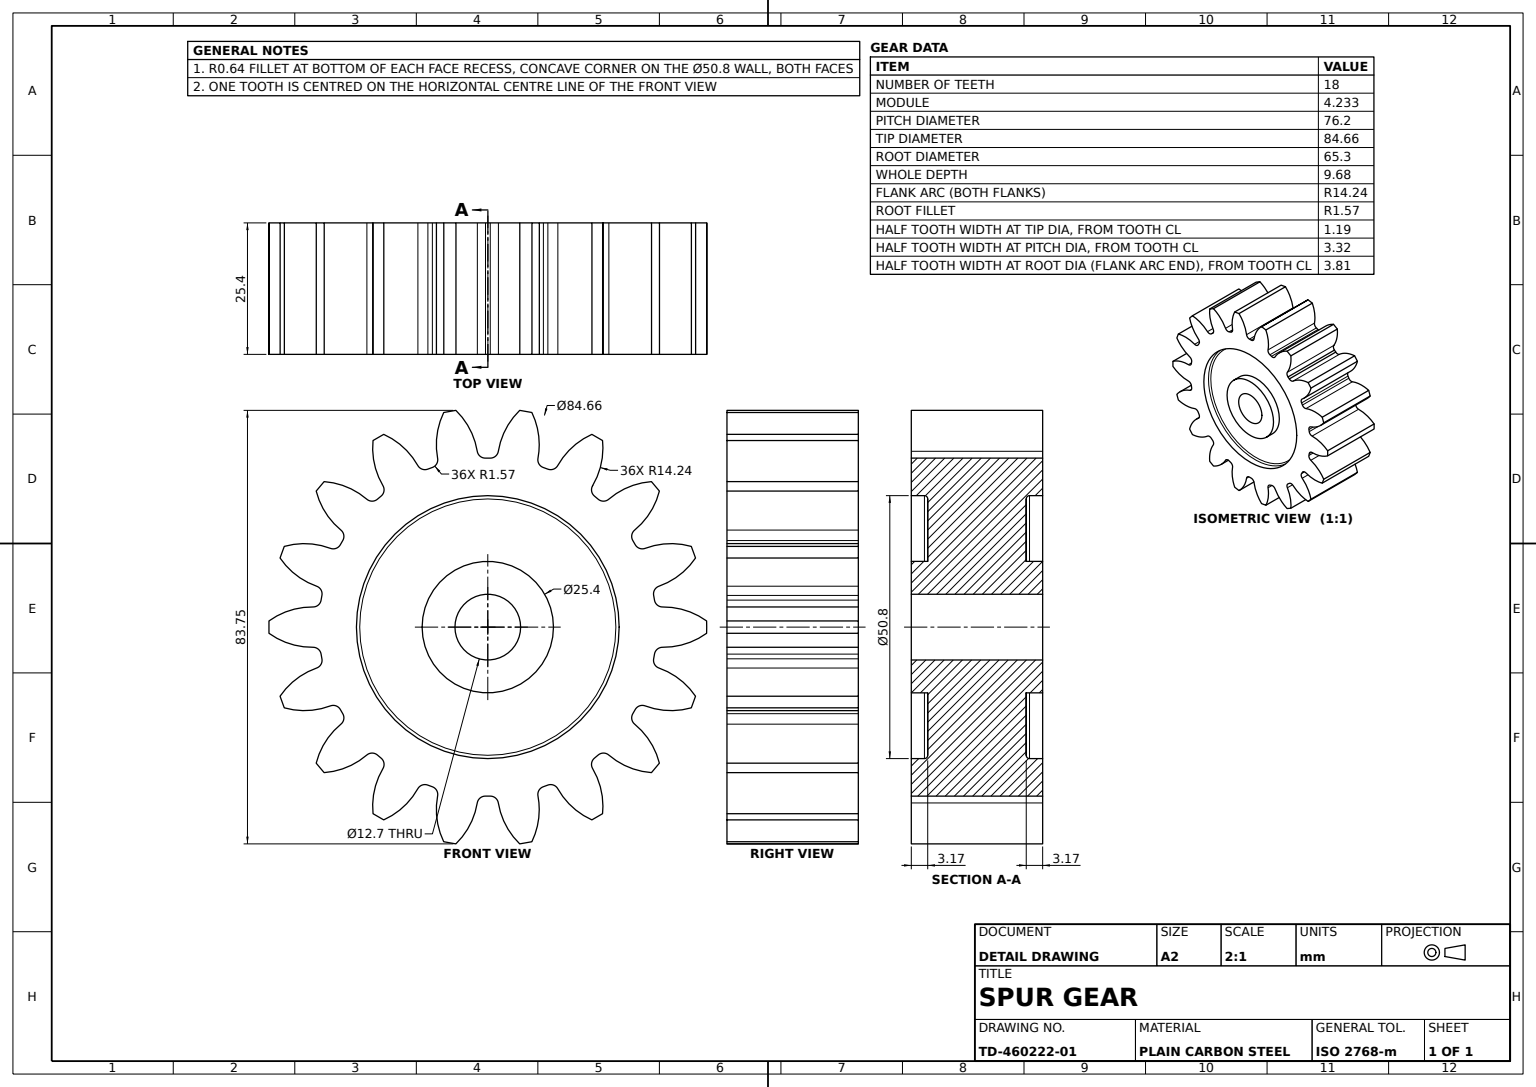
from build123d import *

# Parameters (mm, degrees)
GEAR_PROFILE_18T_SKETCH_R                  = 6.35
GEAR_BODY_18T_DEPTH                        = 12.7
FACE_RECESS_SKETCH_R                       = 25.4
FACE_RECESS_SKETCH_R_2                     = 12.7
FACE_RECESS_0_25IN_DEEP_DEPTH              = 3.175
RECESS_FILLET_R0_025IN_R                   = 0.635
RECESS_FILLET_R0_025IN_OF_FACE_RECESS_MI_R = 0.635


with BuildPart() as part:
    # Gear Profile 18T Sketch → Gear Body 18T (new, symmetric)
    with BuildSketch(Plane.XY):
        with BuildLine():
            ThreePointArc((-42.312262388, 1.1938), (-42.3291, 0), (-42.312262388, -1.1938))
            ThreePointArc((-42.312262388, -1.1938), (-38.27572162, -3.227144912), (-33.805252697, -3.892772818))
            ThreePointArc((-33.805252697, -3.892772818), (-32.773212647, -4.262365971), (-32.232404102, -5.215902483))
            ThreePointArc((-32.232404102, -5.215902483), (-32.155647309, -5.669908203), (-32.072495999, -6.122786396))
            ThreePointArc((-32.072495999, -6.122786396), (-32.254561104, -7.203785037), (-33.09795322, -7.904067481))
            ThreePointArc((-33.09795322, -7.904067481), (-37.071161726, -10.058543535), (-40.168824382, -13.349840996))
            ThreePointArc((-40.168824382, -13.349840996), (-39.776342915, -14.477404849), (-39.352217087, -15.593451097))
            ThreePointArc((-39.352217087, -15.593451097), (-34.863664596, -16.123592054), (-30.435139786, -15.220087264))
            ThreePointArc((-30.435139786, -15.220087264), (-29.338931064, -15.214412737), (-28.50460857, -15.925476545))
            ThreePointArc((-28.50460857, -15.925476545), (-28.277201677, -16.32585), (-28.04417154, -16.722976874))
            ThreePointArc((-28.04417154, -16.722976874), (-27.845533466, -17.801053253), (-28.398552111, -18.74756059))
            ThreePointArc((-28.398552111, -18.74756059), (-31.395272617, -22.131023182), (-33.180433326, -26.283294144))
            ThreePointArc((-33.180433326, -26.283294144), (-32.425971837, -27.208621009), (-31.645713629, -28.112301857))
            ThreePointArc((-31.645713629, -28.112301857), (-27.246535089, -27.075296036), (-23.394099842, -24.711634561))
            ThreePointArc((-23.394099842, -24.711634561), (-22.365941397, -24.331376786), (-21.338736561, -24.7142031))
            ThreePointArc((-21.338736561, -24.7142031), (-20.988108195, -25.012653343), (-20.633306105, -25.306129536))
            ThreePointArc((-20.633306105, -25.306129536), (-20.077923535, -26.251251731), (-20.2738665, -27.329821208))
            ThreePointArc((-20.2738665, -27.329821208), (-21.932650285, -31.534174815), (-22.189992321, -36.046594119))
            ThreePointArc((-22.189992321, -36.046594119), (-21.16455, -36.658075919), (-20.122270067, -37.240394119))
            ThreePointArc((-20.122270067, -37.240394119), (-16.343071335, -34.761319727), (-13.531386197, -31.222594026))
            ThreePointArc((-13.531386197, -31.222594026), (-12.695289112, -30.513617701), (-11.599097997, -30.522032019))
            ThreePointArc((-11.599097997, -30.522032019), (-11.167539114, -30.682561546), (-10.733759438, -30.836989497))
            ThreePointArc((-10.733759438, -30.836989497), (-9.888619707, -31.535161823), (-9.703853378, -32.615702042))
            ThreePointArc((-9.703853378, -32.615702042), (-9.824626637, -37.13383957), (-8.523110752, -41.462142852))
            ThreePointArc((-8.523110752, -41.462142852), (-7.350371077, -41.686025858), (-6.171783761, -41.876745241))
            ThreePointArc((-6.171783761, -41.876745241), (-3.468391979, -38.254615236), (-2.036587675, -33.967647854))
            ThreePointArc((-2.036587675, -33.967647854), (-1.493397598, -33.015465989), (-0.46043703, -32.648453419))
            ThreePointArc((-0.46043703, -32.648453419), (0, -32.6517), (0.46043703, -32.648453419))
            ThreePointArc((0.46043703, -32.648453419), (1.493397598, -33.015465989), (2.036587675, -33.967647854))
            ThreePointArc((2.036587675, -33.967647854), (3.468391979, -38.254615236), (6.171783761, -41.876745241))
            ThreePointArc((6.171783761, -41.876745241), (7.350371077, -41.686025858), (8.523110752, -41.462142852))
            ThreePointArc((8.523110752, -41.462142852), (9.824626637, -37.13383957), (9.703853378, -32.615702042))
            ThreePointArc((9.703853378, -32.615702042), (9.888619707, -31.535161823), (10.733759438, -30.836989497))
            ThreePointArc((10.733759438, -30.836989497), (11.167539114, -30.682561546), (11.599097997, -30.522032019))
            ThreePointArc((11.599097997, -30.522032019), (12.695289112, -30.513617701), (13.531386197, -31.222594026))
            ThreePointArc((13.531386197, -31.222594026), (16.343071335, -34.761319727), (20.122270067, -37.240394119))
            ThreePointArc((20.122270067, -37.240394119), (21.16455, -36.658075919), (22.189992321, -36.046594119))
            ThreePointArc((22.189992321, -36.046594119), (21.932650285, -31.534174815), (20.2738665, -27.329821208))
            ThreePointArc((20.2738665, -27.329821208), (20.077923535, -26.251251731), (20.633306105, -25.306129536))
            ThreePointArc((20.633306105, -25.306129536), (20.988108195, -25.012653343), (21.338736561, -24.7142031))
            ThreePointArc((21.338736561, -24.7142031), (22.365941397, -24.331376786), (23.394099842, -24.711634561))
            ThreePointArc((23.394099842, -24.711634561), (27.246535089, -27.075296036), (31.645713629, -28.112301857))
            ThreePointArc((31.645713629, -28.112301857), (32.425971837, -27.208621009), (33.180433326, -26.283294144))
            ThreePointArc((33.180433326, -26.283294144), (31.395272617, -22.131023182), (28.398552111, -18.74756059))
            ThreePointArc((28.398552111, -18.74756059), (27.845533466, -17.801053253), (28.04417154, -16.722976874))
            ThreePointArc((28.04417154, -16.722976874), (28.277201677, -16.32585), (28.50460857, -15.925476545))
            ThreePointArc((28.50460857, -15.925476545), (29.338931064, -15.214412737), (30.435139786, -15.220087264))
            ThreePointArc((30.435139786, -15.220087264), (34.863664596, -16.123592054), (39.352217087, -15.593451097))
            ThreePointArc((39.352217087, -15.593451097), (39.776342915, -14.477404849), (40.168824382, -13.349840996))
            ThreePointArc((40.168824382, -13.349840996), (37.071161726, -10.058543535), (33.09795322, -7.904067481))
            ThreePointArc((33.09795322, -7.904067481), (32.254561104, -7.203785037), (32.072495999, -6.122786396))
            ThreePointArc((32.072495999, -6.122786396), (32.155647309, -5.669908203), (32.232404102, -5.215902483))
            ThreePointArc((32.232404102, -5.215902483), (32.773212647, -4.262365971), (33.805252697, -3.892772818))
            ThreePointArc((33.805252697, -3.892772818), (38.27572162, -3.227144912), (42.312262388, -1.1938))
            ThreePointArc((42.312262388, -1.1938), (42.3291, 0), (42.312262388, 1.1938))
            ThreePointArc((42.312262388, 1.1938), (38.27572162, 3.227144912), (33.805252697, 3.892772818))
            ThreePointArc((33.805252697, 3.892772818), (32.773212647, 4.262365971), (32.232404102, 5.215902483))
            ThreePointArc((32.232404102, 5.215902483), (32.155647309, 5.669908203), (32.072495999, 6.122786396))
            ThreePointArc((32.072495999, 6.122786396), (32.254561104, 7.203785037), (33.09795322, 7.904067481))
            ThreePointArc((33.09795322, 7.904067481), (37.071161726, 10.058543535), (40.168824382, 13.349840996))
            ThreePointArc((40.168824382, 13.349840996), (39.776342915, 14.477404849), (39.352217087, 15.593451097))
            ThreePointArc((39.352217087, 15.593451097), (34.863664596, 16.123592054), (30.435139786, 15.220087264))
            ThreePointArc((30.435139786, 15.220087264), (29.338931064, 15.214412737), (28.50460857, 15.925476545))
            ThreePointArc((28.50460857, 15.925476545), (28.277201677, 16.32585), (28.04417154, 16.722976874))
            ThreePointArc((28.04417154, 16.722976874), (27.845533466, 17.801053253), (28.398552111, 18.74756059))
            ThreePointArc((28.398552111, 18.74756059), (31.395272617, 22.131023182), (33.180433326, 26.283294144))
            ThreePointArc((33.180433326, 26.283294144), (32.425971837, 27.208621009), (31.645713629, 28.112301857))
            ThreePointArc((31.645713629, 28.112301857), (27.246535089, 27.075296036), (23.394099842, 24.711634561))
            ThreePointArc((23.394099842, 24.711634561), (22.365941397, 24.331376786), (21.338736561, 24.7142031))
            ThreePointArc((21.338736561, 24.7142031), (20.988108195, 25.012653343), (20.633306105, 25.306129536))
            ThreePointArc((20.633306105, 25.306129536), (20.077923535, 26.251251731), (20.2738665, 27.329821208))
            ThreePointArc((20.2738665, 27.329821208), (21.932650285, 31.534174815), (22.189992321, 36.046594119))
            ThreePointArc((22.189992321, 36.046594119), (21.16455, 36.658075919), (20.122270067, 37.240394119))
            ThreePointArc((20.122270067, 37.240394119), (16.343071335, 34.761319727), (13.531386197, 31.222594026))
            ThreePointArc((13.531386197, 31.222594026), (12.695289112, 30.513617701), (11.599097997, 30.522032019))
            ThreePointArc((11.599097997, 30.522032019), (11.167539114, 30.682561546), (10.733759438, 30.836989497))
            ThreePointArc((10.733759438, 30.836989497), (9.888619707, 31.535161823), (9.703853378, 32.615702042))
            ThreePointArc((9.703853378, 32.615702042), (9.824626637, 37.13383957), (8.523110752, 41.462142852))
            ThreePointArc((8.523110752, 41.462142852), (7.350371077, 41.686025858), (6.171783761, 41.876745241))
            ThreePointArc((6.171783761, 41.876745241), (3.468391979, 38.254615236), (2.036587675, 33.967647854))
            ThreePointArc((2.036587675, 33.967647854), (1.493397598, 33.015465989), (0.46043703, 32.648453419))
            ThreePointArc((0.46043703, 32.648453419), (0, 32.6517), (-0.46043703, 32.648453419))
            ThreePointArc((-0.46043703, 32.648453419), (-1.493397598, 33.015465989), (-2.036587675, 33.967647854))
            ThreePointArc((-2.036587675, 33.967647854), (-3.468391979, 38.254615236), (-6.171783761, 41.876745241))
            ThreePointArc((-6.171783761, 41.876745241), (-7.350371077, 41.686025858), (-8.523110752, 41.462142852))
            ThreePointArc((-8.523110752, 41.462142852), (-9.824626637, 37.13383957), (-9.703853378, 32.615702042))
            ThreePointArc((-9.703853378, 32.615702042), (-9.888619707, 31.535161823), (-10.733759438, 30.836989497))
            ThreePointArc((-10.733759438, 30.836989497), (-11.167539114, 30.682561546), (-11.599097997, 30.522032019))
            ThreePointArc((-11.599097997, 30.522032019), (-12.695289112, 30.513617701), (-13.531386197, 31.222594026))
            ThreePointArc((-13.531386197, 31.222594026), (-16.343071335, 34.761319727), (-20.122270067, 37.240394119))
            ThreePointArc((-20.122270067, 37.240394119), (-21.16455, 36.658075919), (-22.189992321, 36.046594119))
            ThreePointArc((-22.189992321, 36.046594119), (-21.932650285, 31.534174815), (-20.2738665, 27.329821208))
            ThreePointArc((-20.2738665, 27.329821208), (-20.077923535, 26.251251731), (-20.633306105, 25.306129536))
            Line((-20.633306105, 25.306129536), (-21.338736561, 24.7142031))
            ThreePointArc((-21.338736561, 24.7142031), (-22.365941397, 24.331376786), (-23.394099842, 24.711634561))
            ThreePointArc((-23.394099842, 24.711634561), (-27.246535089, 27.075296036), (-31.645713629, 28.112301857))
            ThreePointArc((-31.645713629, 28.112301857), (-32.425971837, 27.208621009), (-33.180433326, 26.283294144))
            ThreePointArc((-33.180433326, 26.283294144), (-31.395272617, 22.131023182), (-28.398552111, 18.74756059))
            ThreePointArc((-28.398552111, 18.74756059), (-27.845533466, 17.801053253), (-28.04417154, 16.722976874))
            ThreePointArc((-28.04417154, 16.722976874), (-28.277201677, 16.32585), (-28.50460857, 15.925476545))
            ThreePointArc((-28.50460857, 15.925476545), (-29.338931064, 15.214412737), (-30.435139786, 15.220087264))
            ThreePointArc((-30.435139786, 15.220087264), (-34.863664596, 16.123592054), (-39.352217087, 15.593451097))
            ThreePointArc((-39.352217087, 15.593451097), (-39.776342915, 14.477404849), (-40.168824382, 13.349840996))
            ThreePointArc((-40.168824382, 13.349840996), (-37.071161726, 10.058543535), (-33.09795322, 7.904067481))
            ThreePointArc((-33.09795322, 7.904067481), (-32.254561104, 7.203785037), (-32.072495999, 6.122786396))
            ThreePointArc((-32.072495999, 6.122786396), (-32.155647309, 5.669908203), (-32.232404102, 5.215902483))
            ThreePointArc((-32.232404102, 5.215902483), (-32.773212647, 4.262365971), (-33.805252697, 3.892772818))
            ThreePointArc((-33.805252697, 3.892772818), (-38.27572162, 3.227144912), (-42.312262388, 1.1938))
        make_face()
        Circle(GEAR_PROFILE_18T_SKETCH_R, mode=Mode.SUBTRACT)
    extrude(amount=GEAR_BODY_18T_DEPTH, both=True)

    # Face Recess Sketch → Face Recess 0.25in Deep (cut, symmetric)
    with BuildSketch(Plane(origin=(0, 0, -12.7), x_dir=(-1, 0, 0), z_dir=(0, 0, -1))):
        Circle(FACE_RECESS_SKETCH_R)
        Circle(FACE_RECESS_SKETCH_R_2, mode=Mode.SUBTRACT)
    face_recess_0_25in_deep = extrude(amount=FACE_RECESS_0_25IN_DEEP_DEPTH, both=True, mode=Mode.SUBTRACT)

    # Recess Fillet R0.025in
    recess_fillet_r0_025in_edges = [part.edges().sort_by_distance(p)[0] for p in [
        (25.4, 0, -9.525),
    ]]
    fillet(recess_fillet_r0_025in_edges, radius=RECESS_FILLET_R0_025IN_R)

    # Face Recess Mirror: Face Recess 0.25in Deep across plane
    add(face_recess_0_25in_deep.mirror(Plane.XY), mode=Mode.SUBTRACT)

    # Recess Fillet R0.025in of Face Recess Mi
    recess_fillet_r0_025in_of_face_recess_mi_edges = [part.edges().sort_by_distance(p)[0] for p in [
        (25.4, 0, 9.525),
    ]]
    fillet(recess_fillet_r0_025in_of_face_recess_mi_edges, radius=RECESS_FILLET_R0_025IN_OF_FACE_RECESS_MI_R)


solid = part.part
